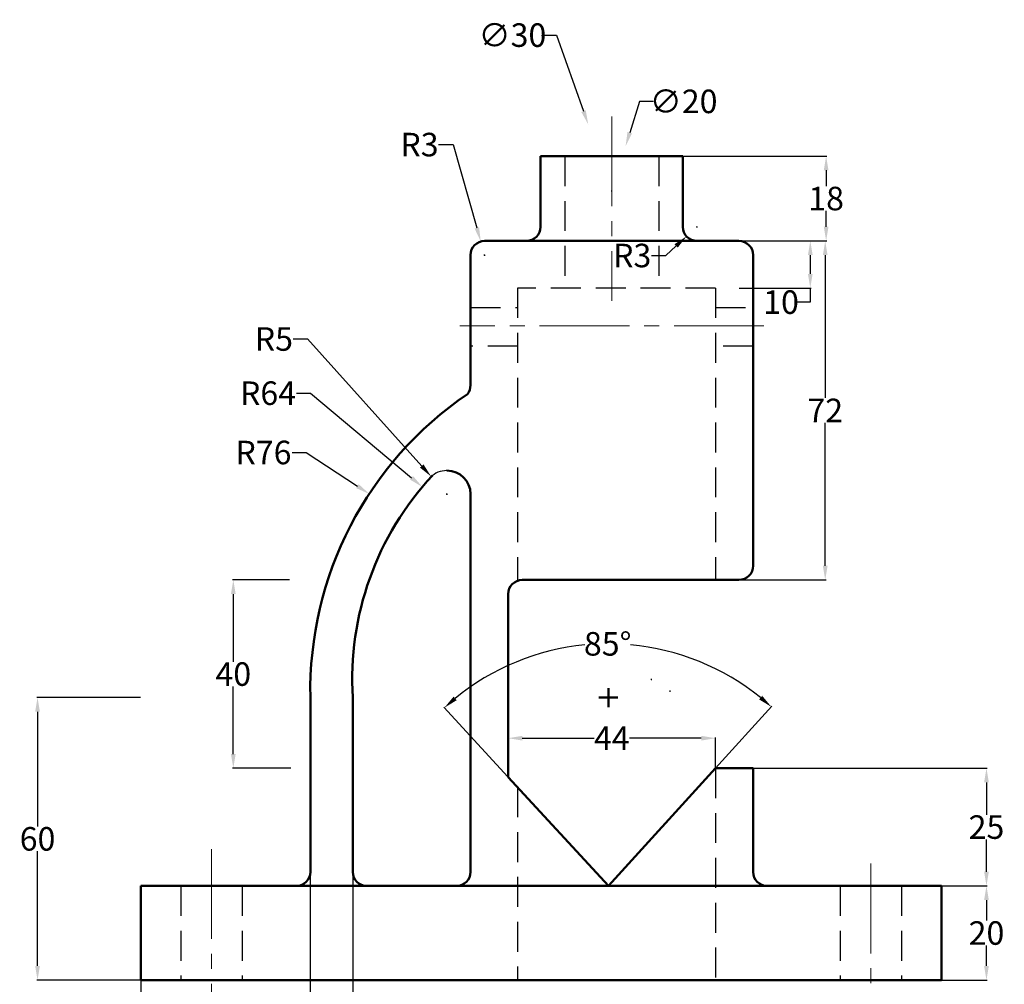
# Model space of a CAD drawing. Units: metres. Extents: x -2793 to -2360, y -31 to 491.
# Tile 2 of 4: x -2786 to -2577, y 144 to 349. Entities that reach past the tile are written whole.
import ezdxf

# ---------------------------------------------------------------- set-up
doc = ezdxf.new("R2010")
doc.units = ezdxf.units.M
doc.linetypes.add('CENTER2', pattern=[28.575, 19.05, -3.175, 3.175, -3.175])
doc.linetypes.add('DASHED2', pattern=[9.525, 6.35, -3.175])
for name, color, linetype, lineweight in [('M-CNTR', 9, 'CENTER2', 18), ('M-DIMS', 2, 'Continuous', 25), ('M-HIDN', 9, 'DASHED2', 25), ('M-OUTL', 7, 'Continuous', 50)]:
    doc.layers.add(name, color=color, linetype=linetype, lineweight=lineweight)
doc.styles.get("Standard").update_dxf_attribs({"font": 'arial.ttf'})
doc.dimstyles.get("Standard").update_dxf_attribs({"dimtxt": 5, "dimasz": 3, "dimexe": 0.18, "dimexo": 0.0625, "dimgap": 0.09, "dimtad": 0, "dimtih": 1, "dimtoh": 1, "dimdec": 0, "dimzin": 0, "dimdsep": 46, "dimtxsty": 'Standard', "dimcen": 0.09, "dimclrd": 254, "dimclre": 254, "dimadec": 0, "dimazin": 0, "dimtfac": 1, "dimtdec": 0, "dimtofl": 0, "dimtmove": 0, "dimatfit": 3, "dimfxl": 1, "dimtolj": 1, "dimtzin": 0, "dimarcsym": 0})

# ---------------------------------------------------------------- blocks, each defined once
blk = doc.blocks.new('*D15')
at = {"layer": 'Defpoints', "color": 0, "transparency": 16777216}
for p in [(-2648.17, 215.08), (-2681.87, 188.31), (-2637.87, 190.18), (-2660.6, 165.18), (-2660.6, 165.18)]:
    blk.add_point(p, dxfattribs=at)
at = {"layer": 'M-DIMS', "color": 0, "lineweight": -2, "transparency": 16777216}
for p, q in [((-2681.91, 188.36), (-2695.53, 203.17)), ((-2637.83, 190.22), (-2625.88, 203.36))]:
    blk.add_line(p, q, dxfattribs=at)
for start, end in [(95.5587, 129.2471), (51.0616, 84.7514)]:
    blk.add_arc((-2660.6, 165.18), 51.43, start, end, dxfattribs=at)
at = {"layer": 'M-DIMS', "color": 0, "transparency": 16777216}
for points in [[(-2692.81, 204.62), (-2693.47, 205.38), (-2695.4, 203.04)], [(-2627.95, 205.56), (-2628.6, 204.8), (-2626, 203.22)]]:
    blk.add_solid(points, dxfattribs=at)
at = {"layer": 'M-DIMS', "color": 0, "transparency": 16777216, "insert": (-2660.74, 216.6), "char_height": 5, "attachment_point": 5}
blk.add_mtext('\\A1;{\\fTimes New Roman|b0|i0|c0|p18;85°}', dxfattribs=at)
blk = doc.blocks.new('*D16')
at = {"layer": 'Defpoints', "color": 0, "transparency": 16777216}
for p in [(-2781.78, 205.18), (-2759.87, 205.18), (-2759.87, 145.18)]:
    blk.add_point(p, dxfattribs=at)
at = {"layer": 'M-DIMS', "color": 0, "lineweight": -2, "transparency": 16777216}
for p, q in [((-2759.93, 205.18), (-2781.96, 205.18)), ((-2781.78, 202.18), (-2781.78, 177.81)), ((-2781.78, 148.18), (-2781.78, 172.54)), ((-2759.93, 145.18), (-2781.96, 145.18))]:
    blk.add_line(p, q, dxfattribs=at)
at = {"layer": 'M-DIMS', "color": 0, "transparency": 16777216}
for points in [[(-2782.28, 202.18), (-2781.28, 202.18), (-2781.78, 205.18)], [(-2782.28, 148.18), (-2781.28, 148.18), (-2781.78, 145.18)]]:
    blk.add_solid(points, dxfattribs=at)
at = {"layer": 'M-DIMS', "color": 0, "transparency": 16777216, "insert": (-2781.78, 175.18), "char_height": 5, "attachment_point": 5}
blk.add_mtext('\\A1;{\\fTimes New Roman|b0|i0|c0|p18;60}', dxfattribs=at)
blk = doc.blocks.new('*D17')
at = {"layer": 'Defpoints', "color": 0, "transparency": 16777216}
for p in [(-2656.94, 322.3), (-2662.8, 303.26)]:
    blk.add_point(p, dxfattribs=at)
at = {"layer": 'M-DIMS', "color": 0, "lineweight": -2, "transparency": 16777216}
for p, q in [((-2654.01, 331.82), (-2656.06, 325.17)), ((-2651.01, 331.82), (-2654.01, 331.82)), ((-2659.96, 312.78), (-2659.78, 312.78)), ((-2659.87, 312.69), (-2659.87, 312.87))]:
    blk.add_line(p, q, dxfattribs=at)
at = {"layer": 'M-DIMS', "color": 0, "transparency": 16777216}
blk.add_solid([(-2656.54, 325.32), (-2655.58, 325.02), (-2656.94, 322.3)], dxfattribs=at)
at = {"layer": 'M-DIMS', "color": 0, "transparency": 16777216, "insert": (-2644.63, 331.82), "char_height": 5, "attachment_point": 5}
blk.add_mtext('\\A1;∅20', dxfattribs=at)
blk = doc.blocks.new('*D18')
at = {"layer": 'Defpoints', "color": 0, "transparency": 16777216}
for p in [(-2664.87, 326.92), (-2654.87, 298.64)]:
    blk.add_point(p, dxfattribs=at)
at = {"layer": 'M-DIMS', "color": 0, "lineweight": -2, "transparency": 16777216}
for p, q in [((-2674.78, 345.89), (-2671.58, 345.89)), ((-2671.58, 345.89), (-2665.87, 329.75)), ((-2659.96, 312.78), (-2659.78, 312.78)), ((-2659.87, 312.69), (-2659.87, 312.87))]:
    blk.add_line(p, q, dxfattribs=at)
at = {"layer": 'M-DIMS', "color": 0, "transparency": 16777216}
blk.add_solid([(-2665.4, 329.91), (-2666.34, 329.58), (-2664.87, 326.92)], dxfattribs=at)
at = {"layer": 'M-DIMS', "color": 0, "transparency": 16777216, "insert": (-2680.97, 345.89), "char_height": 5, "attachment_point": 5}
blk.add_mtext('\\A1;{\\fTimes New Roman|b0|i0|c0|p18;∅30}', dxfattribs=at)
blk = doc.blocks.new('*D19')
at = {"layer": 'Defpoints', "color": 0, "transparency": 16777216}
for p in [(-2687.69, 302.06), (-2686.87, 299.18)]:
    blk.add_point(p, dxfattribs=at)
at = {"layer": 'M-DIMS', "color": 0, "lineweight": -2, "transparency": 16777216}
for p, q in [((-2696.67, 322.64), (-2693.57, 322.64)), ((-2693.57, 322.64), (-2688.52, 304.94)), ((-2686.96, 299.18), (-2686.78, 299.18)), ((-2686.87, 299.09), (-2686.87, 299.27))]:
    blk.add_line(p, q, dxfattribs=at)
at = {"layer": 'M-DIMS', "color": 0, "transparency": 16777216}
blk.add_solid([(-2688.04, 305.08), (-2689, 304.81), (-2687.69, 302.06)], dxfattribs=at)
at = {"layer": 'M-DIMS', "color": 0, "transparency": 16777216, "insert": (-2700.7, 322.64), "char_height": 5, "attachment_point": 5}
blk.add_mtext('\\A1;{\\fTimes New Roman|b0|i0|c0|p18;R3}', dxfattribs=at)
blk = doc.blocks.new('*D20')
at = {"layer": 'Defpoints', "color": 0, "transparency": 16777216}
for p in [(-2698.21, 252.13), (-2694.87, 248.41)]:
    blk.add_point(p, dxfattribs=at)
at = {"layer": 'M-DIMS', "color": 0, "lineweight": -2, "transparency": 16777216}
for p, q in [((-2727.52, 281.35), (-2724.47, 281.35)), ((-2724.47, 281.35), (-2700.21, 254.36)), ((-2694.96, 248.41), (-2694.78, 248.41)), ((-2694.87, 248.32), (-2694.87, 248.5))]:
    blk.add_line(p, q, dxfattribs=at)
blk.add_arc((-2694.87, 248.41), 5, 90.7162, 134.0032, dxfattribs=at)
at = {"layer": 'M-DIMS', "color": 0, "transparency": 16777216}
blk.add_solid([(-2699.84, 254.7), (-2700.59, 254.03), (-2698.21, 252.13)], dxfattribs=at)
at = {"layer": 'M-DIMS', "color": 0, "transparency": 16777216, "insert": (-2731.61, 281.35), "char_height": 5, "attachment_point": 5}
blk.add_mtext('\\A1;{\\fTimes New Roman|b0|i0|c0|p18;R5}', dxfattribs=at)
blk = doc.blocks.new('*D21')
at = {"layer": 'Defpoints', "color": 0, "transparency": 16777216}
for p in [(-2711.37, 248.45), (-2647.51, 206.57)]:
    blk.add_point(p, dxfattribs=at)
at = {"layer": 'M-DIMS', "color": 0, "lineweight": -2, "transparency": 16777216}
for p, q in [((-2727.76, 257.24), (-2724.76, 257.24)), ((-2724.76, 257.24), (-2713.88, 250.1)), ((-2647.6, 206.57), (-2647.42, 206.57)), ((-2647.51, 206.48), (-2647.51, 206.66))]:
    blk.add_line(p, q, dxfattribs=at)
at = {"layer": 'M-DIMS', "color": 0, "transparency": 16777216}
blk.add_solid([(-2713.6, 250.52), (-2714.15, 249.68), (-2711.37, 248.45)], dxfattribs=at)
at = {"layer": 'M-DIMS', "color": 0, "transparency": 16777216, "insert": (-2733.82, 257.24), "char_height": 5, "attachment_point": 5}
blk.add_mtext('\\A1;R76', dxfattribs=at)
blk = doc.blocks.new('*D22')
at = {"layer": 'Defpoints', "color": 0, "transparency": 16777216}
for p in [(-2700.09, 249.93), (-2651.44, 209.05)]:
    blk.add_point(p, dxfattribs=at)
at = {"layer": 'M-DIMS', "color": 0, "lineweight": -2, "transparency": 16777216}
for p, q in [((-2726.8, 269.84), (-2723.8, 269.84)), ((-2723.8, 269.84), (-2702.39, 251.86)), ((-2651.53, 209.05), (-2651.35, 209.05)), ((-2651.44, 208.96), (-2651.44, 209.14))]:
    blk.add_line(p, q, dxfattribs=at)
at = {"layer": 'M-DIMS', "color": 0, "transparency": 16777216}
blk.add_solid([(-2702.07, 252.24), (-2702.71, 251.48), (-2700.09, 249.93)], dxfattribs=at)
at = {"layer": 'M-DIMS', "color": 0, "transparency": 16777216, "insert": (-2732.85, 269.84), "char_height": 5, "attachment_point": 5}
blk.add_mtext('\\A1;R64', dxfattribs=at)
blk = doc.blocks.new('*D23')
at = {"layer": 'Defpoints', "color": 0, "transparency": 16777216}
for p in [(-2728.24, 230.18), (-2740.22, 190.18), (-2727.94, 190.18)]:
    blk.add_point(p, dxfattribs=at)
at = {"layer": 'M-DIMS', "color": 0, "lineweight": -2, "transparency": 16777216}
for p, q in [((-2728.3, 230.18), (-2740.4, 230.18)), ((-2740.22, 227.18), (-2740.22, 212.81)), ((-2740.22, 193.18), (-2740.22, 207.54)), ((-2728, 190.18), (-2740.4, 190.18))]:
    blk.add_line(p, q, dxfattribs=at)
at = {"layer": 'M-DIMS', "color": 0, "transparency": 16777216}
for points in [[(-2740.72, 227.18), (-2739.72, 227.18), (-2740.22, 230.18)], [(-2740.72, 193.18), (-2739.72, 193.18), (-2740.22, 190.18)]]:
    blk.add_solid(points, dxfattribs=at)
at = {"layer": 'M-DIMS', "color": 0, "transparency": 16777216, "insert": (-2740.22, 210.18), "char_height": 5, "attachment_point": 5}
blk.add_mtext('\\A1;{\\fTimes New Roman|b0|i0|c0|p18;40}', dxfattribs=at)
blk = doc.blocks.new('*D24')
at = {"layer": 'Defpoints', "color": 0, "transparency": 16777216}
for p in [(-2681.87, 196.56), (-2681.87, 188.31), (-2637.87, 190.18)]:
    blk.add_point(p, dxfattribs=at)
at = {"layer": 'M-DIMS', "color": 0, "lineweight": -2, "transparency": 16777216}
for p, q in [((-2681.87, 188.37), (-2681.87, 196.74)), ((-2678.87, 196.56), (-2663.63, 196.56)), ((-2640.87, 196.56), (-2656.11, 196.56)), ((-2637.87, 190.24), (-2637.87, 196.74))]:
    blk.add_line(p, q, dxfattribs=at)
at = {"layer": 'M-DIMS', "color": 0, "transparency": 16777216}
for points in [[(-2678.87, 197.06), (-2678.87, 196.06), (-2681.87, 196.56)], [(-2640.87, 197.06), (-2640.87, 196.06), (-2637.87, 196.56)]]:
    blk.add_solid(points, dxfattribs=at)
at = {"layer": 'M-DIMS', "color": 0, "transparency": 16777216, "insert": (-2659.87, 196.56), "char_height": 5, "attachment_point": 5}
blk.add_mtext('\\A1;44', dxfattribs=at)
blk = doc.blocks.new('*D25')
at = {"layer": 'Defpoints', "color": 0, "transparency": 16777216}
for p in [(-2589.87, 165.18), (-2589.87, 145.18), (-2580.33, 145.18)]:
    blk.add_point(p, dxfattribs=at)
at = {"layer": 'M-DIMS', "color": 0, "lineweight": -2, "transparency": 16777216}
for p, q in [((-2589.81, 165.18), (-2580.15, 165.18)), ((-2580.33, 162.18), (-2580.33, 157.81)), ((-2580.33, 148.18), (-2580.33, 152.54)), ((-2589.81, 145.18), (-2580.15, 145.18))]:
    blk.add_line(p, q, dxfattribs=at)
at = {"layer": 'M-DIMS', "color": 0, "transparency": 16777216}
for points in [[(-2580.83, 162.18), (-2579.83, 162.18), (-2580.33, 165.18)], [(-2580.83, 148.18), (-2579.83, 148.18), (-2580.33, 145.18)]]:
    blk.add_solid(points, dxfattribs=at)
at = {"layer": 'M-DIMS', "color": 0, "transparency": 16777216, "insert": (-2580.33, 155.18), "char_height": 5, "attachment_point": 5}
blk.add_mtext('\\A1;{\\fTimes New Roman|b0|i0|c0|p18;20}', dxfattribs=at)
blk = doc.blocks.new('*D26')
at = {"layer": 'Defpoints', "color": 0, "transparency": 16777216}
for p in [(-2629.87, 190.18), (-2629.87, 165.18), (-2580.33, 165.18)]:
    blk.add_point(p, dxfattribs=at)
at = {"layer": 'M-DIMS', "color": 0, "lineweight": -2, "transparency": 16777216}
for p, q in [((-2629.81, 190.18), (-2580.15, 190.18)), ((-2580.33, 187.18), (-2580.33, 180.31)), ((-2580.33, 168.18), (-2580.33, 175.04)), ((-2629.81, 165.18), (-2580.15, 165.18))]:
    blk.add_line(p, q, dxfattribs=at)
at = {"layer": 'M-DIMS', "color": 0, "transparency": 16777216}
for points in [[(-2580.83, 187.18), (-2579.83, 187.18), (-2580.33, 190.18)], [(-2580.83, 168.18), (-2579.83, 168.18), (-2580.33, 165.18)]]:
    blk.add_solid(points, dxfattribs=at)
at = {"layer": 'M-DIMS', "color": 0, "transparency": 16777216, "insert": (-2580.33, 177.68), "char_height": 5, "attachment_point": 5}
blk.add_mtext('\\A1;{\\fTimes New Roman|b0|i0|c0|p18;25}', dxfattribs=at)
blk = doc.blocks.new('*D27')
at = {"layer": 'Defpoints', "color": 0, "transparency": 16777216}
for p in [(-2632.87, 302.18), (-2632.87, 292.18), (-2617.73, 292.18)]:
    blk.add_point(p, dxfattribs=at)
at = {"layer": 'M-DIMS', "color": 0, "lineweight": -2, "transparency": 16777216}
for p, q in [((-2632.81, 302.18), (-2617.55, 302.18)), ((-2617.73, 299.18), (-2617.73, 295.18)), ((-2632.81, 292.18), (-2617.55, 292.18)), ((-2617.73, 292.18), (-2617.73, 289.18)), ((-2617.73, 289.18), (-2620.73, 289.18))]:
    blk.add_line(p, q, dxfattribs=at)
at = {"layer": 'M-DIMS', "color": 0, "transparency": 16777216}
for points in [[(-2618.23, 299.18), (-2617.23, 299.18), (-2617.73, 302.18)], [(-2618.23, 295.18), (-2617.23, 295.18), (-2617.73, 292.18)]]:
    blk.add_solid(points, dxfattribs=at)
at = {"layer": 'M-DIMS', "color": 0, "transparency": 16777216, "insert": (-2623.94, 289.18), "char_height": 5, "attachment_point": 5}
blk.add_mtext('\\A1;{\\fTimes New Roman|b0|i0|c0|p18;10}', dxfattribs=at)
blk = doc.blocks.new('*D28')
at = {"layer": 'Defpoints', "color": 0, "transparency": 16777216}
for p in [(-2644.8, 320.18), (-2644.8, 302.18), (-2614.37, 302.18)]:
    blk.add_point(p, dxfattribs=at)
at = {"layer": 'M-DIMS', "color": 0, "lineweight": -2, "transparency": 16777216}
for p, q in [((-2644.74, 320.18), (-2614.19, 320.18)), ((-2614.37, 317.18), (-2614.37, 313.81)), ((-2614.37, 305.18), (-2614.37, 308.54)), ((-2644.74, 302.18), (-2614.19, 302.18))]:
    blk.add_line(p, q, dxfattribs=at)
at = {"layer": 'M-DIMS', "color": 0, "transparency": 16777216}
for points in [[(-2614.87, 317.18), (-2613.87, 317.18), (-2614.37, 320.18)], [(-2614.87, 305.18), (-2613.87, 305.18), (-2614.37, 302.18)]]:
    blk.add_solid(points, dxfattribs=at)
at = {"layer": 'M-DIMS', "color": 0, "transparency": 16777216, "insert": (-2614.37, 311.18), "char_height": 5, "attachment_point": 5}
blk.add_mtext('\\A1;{\\fTimes New Roman|b0|i0|c0|p18;18}', dxfattribs=at)
blk = doc.blocks.new('*D29')
at = {"layer": 'Defpoints', "color": 0, "transparency": 16777216}
for p in [(-2632.87, 302.18), (-2632.87, 230.18), (-2614.56, 230.18)]:
    blk.add_point(p, dxfattribs=at)
at = {"layer": 'M-DIMS', "color": 0, "lineweight": -2, "transparency": 16777216}
for p, q in [((-2632.81, 302.18), (-2614.38, 302.18)), ((-2614.56, 299.18), (-2614.56, 268.82)), ((-2614.56, 233.18), (-2614.56, 263.53)), ((-2632.81, 230.18), (-2614.38, 230.18))]:
    blk.add_line(p, q, dxfattribs=at)
at = {"layer": 'M-DIMS', "color": 0, "transparency": 16777216}
for points in [[(-2615.06, 299.18), (-2614.06, 299.18), (-2614.56, 302.18)], [(-2615.06, 233.18), (-2614.06, 233.18), (-2614.56, 230.18)]]:
    blk.add_solid(points, dxfattribs=at)
at = {"layer": 'M-DIMS', "color": 0, "transparency": 16777216, "insert": (-2614.56, 266.18), "char_height": 5, "attachment_point": 5}
blk.add_mtext('\\A1;{\\fTimes New Roman|b0|i0|c0|p18;72}', dxfattribs=at)
blk = doc.blocks.new('*D56')
at = {"layer": 'Defpoints', "color": 0, "transparency": 16777216}
for p in [(-2723.87, 168.18), (-2759.87, 145.18), (-2723.87, 121.23)]:
    blk.add_point(p, dxfattribs=at)
at = {"layer": 'M-DIMS', "color": 254, "lineweight": -2, "transparency": 16777216}
for p, q in [((-2723.87, 168.11), (-2723.87, 121.05)), ((-2759.87, 145.11), (-2759.87, 121.05)), ((-2756.87, 121.23), (-2745.54, 121.23)), ((-2726.87, 121.23), (-2738.2, 121.23))]:
    blk.add_line(p, q, dxfattribs=at)
at = {"layer": 'M-DIMS', "color": 254, "transparency": 16777216}
for points in [[(-2756.87, 121.73), (-2756.87, 120.73), (-2759.87, 121.23)], [(-2726.87, 121.73), (-2726.87, 120.73), (-2723.87, 121.23)]]:
    blk.add_solid(points, dxfattribs=at)
at = {"layer": 'M-DIMS', "color": 0, "transparency": 16777216, "insert": (-2741.87, 121.23), "char_height": 5, "attachment_point": 5}
blk.add_mtext('\\A1;36', dxfattribs=at)
blk = doc.blocks.new('*D57')
at = {"layer": 'Defpoints', "color": 0, "transparency": 16777216}
for p in [(-2723.87, 168.18), (-2714.87, 168.18), (-2714.87, 121.23)]:
    blk.add_point(p, dxfattribs=at)
at = {"layer": 'M-DIMS', "color": 254, "lineweight": -2, "transparency": 16777216}
for p, q in [((-2723.87, 168.11), (-2723.87, 121.05)), ((-2714.87, 168.11), (-2714.87, 121.05)), ((-2720.87, 121.23), (-2717.87, 121.23)), ((-2714.87, 121.23), (-2711.87, 121.23))]:
    blk.add_line(p, q, dxfattribs=at)
at = {"layer": 'M-DIMS', "color": 254, "transparency": 16777216}
for points in [[(-2720.87, 121.73), (-2720.87, 120.73), (-2723.87, 121.23)], [(-2717.87, 121.73), (-2717.87, 120.73), (-2714.87, 121.23)]]:
    blk.add_solid(points, dxfattribs=at)
at = {"layer": 'M-DIMS', "color": 0, "transparency": 16777216, "insert": (-2710.13, 121.23), "char_height": 5, "attachment_point": 5}
blk.add_mtext('\\A1;9', dxfattribs=at)
blk = doc.blocks.new('*D68')
at = {"layer": 'Defpoints', "color": 0, "transparency": 16777216}
for p in [(-2641.8, 305.18), (-2644.01, 303.15)]:
    blk.add_point(p, dxfattribs=at)
at = {"layer": 'M-DIMS', "color": 254, "lineweight": -2, "transparency": 16777216}
for p, q in [((-2641.89, 305.18), (-2641.71, 305.18)), ((-2641.8, 305.09), (-2641.8, 305.27)), ((-2648.42, 299.08), (-2646.21, 301.11)), ((-2651.42, 299.08), (-2648.42, 299.08))]:
    blk.add_line(p, q, dxfattribs=at)
at = {"layer": 'M-DIMS', "color": 254, "transparency": 16777216}
blk.add_solid([(-2646.55, 301.48), (-2645.88, 300.75), (-2644.01, 303.15)], dxfattribs=at)
at = {"layer": 'M-DIMS', "color": 0, "transparency": 16777216, "insert": (-2655.54, 299.08), "char_height": 5, "attachment_point": 5}
blk.add_mtext('\\A1;R3', dxfattribs=at)

msp = doc.modelspace()

# ---------------------------------------------------------------- linework, layer by layer
at = {"layer": 'M-CNTR'}
for p, q in [((-2659.868, 328.595), (-2659.868, 289.42)), ((-2627.566, 284.142), (-2692.115, 284.142)), ((-2744.868, 172.975), (-2744.868, 136.879)), ((-2604.868, 169.913), (-2604.868, 140.718))]:
    msp.add_line(p, q, dxfattribs=at)
at = {"layer": 'M-HIDN'}
for p, q in [((-2669.868, 320.175), (-2669.868, 292.175)), ((-2649.868, 320.175), (-2649.868, 292.175)), ((-2637.868, 292.175), (-2679.868, 292.175)), ((-2679.868, 292.175), (-2679.868, 230.004)), ((-2637.868, 292.175), (-2637.868, 230.175)), ((-2689.868, 288.016), (-2679.868, 288.016)), ((-2637.868, 288.016), (-2629.868, 288.016)), ((-2679.868, 279.796), (-2689.868, 279.796)), ((-2629.868, 279.796), (-2637.868, 279.796)), ((-2637.868, 190.175), (-2637.868, 145.175)), ((-2679.868, 186.135), (-2679.868, 145.175)), ((-2751.368, 165.175), (-2751.368, 145.175)), ((-2738.368, 165.175), (-2738.368, 145.175)), ((-2611.368, 165.175), (-2611.368, 145.175)), ((-2598.368, 165.175), (-2598.368, 145.175))]:
    msp.add_line(p, q, dxfattribs=at)
at = {"layer": 'M-OUTL'}
for p, q in [((-2644.798, 320.175), (-2674.999, 320.175)), ((-2674.999, 320.175), (-2674.999, 305.175)), ((-2644.798, 320.175), (-2644.798, 305.175)), ((-2677.999, 302.175), (-2686.868, 302.175)), ((-2677.999, 302.175), (-2641.798, 302.175)), ((-2632.868, 302.175), (-2641.798, 302.175)), ((-2689.868, 299.175), (-2689.868, 271.546)), ((-2629.868, 299.175), (-2629.868, 233.175)), ((-2689.868, 248.411), (-2689.868, 168.175)), ((-2632.868, 230.175), (-2678.868, 230.175)), ((-2681.868, 227.175), (-2681.868, 188.311)), ((-2660.601, 205.175), (-2660.601, 207.175)), ((-2660.601, 207.175), (-2660.601, 203.175)), ((-2723.868, 205.175), (-2723.868, 168.175)), ((-2714.868, 205.175), (-2714.868, 168.175)), ((-2658.601, 205.175), (-2662.601, 205.175)), ((-2660.601, 205.175), (-2658.601, 205.175)), ((-2681.868, 188.311), (-2660.601, 165.175)), ((-2660.601, 165.175), (-2637.868, 190.175)), ((-2629.868, 190.175), (-2637.868, 190.175)), ((-2629.868, 190.175), (-2629.868, 168.175)), ((-2759.868, 165.175), (-2759.868, 145.175)), ((-2726.868, 165.175), (-2759.868, 165.175)), ((-2726.868, 165.175), (-2711.868, 165.175)), ((-2692.868, 165.175), (-2711.868, 165.175)), ((-2626.868, 165.175), (-2692.868, 165.175)), ((-2589.868, 165.175), (-2626.868, 165.175)), ((-2589.868, 145.175), (-2589.868, 165.175)), ((-2759.868, 145.175), (-2589.868, 145.175))]:
    msp.add_line(p, q, dxfattribs=at)
for centre, radius, start, end in [((-2677.999, 305.175), 3, 270, 0), ((-2641.798, 305.175), 3, 180, 270), ((-2686.868, 299.175), 3, 90, 180), ((-2632.868, 299.175), 3, 360, 90), ((-2647.512, 206.565), 76.368, 124.2849, 181.04273), ((-2692.868, 271.546), 3, 321.16359, 0), ((-2694.868, 248.411), 5, 0, 90), ((-2651.44, 209.05), 63.546, 137.06049, 183.4962), ((-2632.868, 233.175), 3, 270, 360), ((-2678.868, 227.175), 3, 90, 180), ((-2726.868, 168.175), 3, 270, 0), ((-2711.868, 168.175), 3, 180, 270), ((-2692.868, 168.175), 3, 270, 0), ((-2626.868, 168.175), 3, 180, 270)]:
    msp.add_arc(centre, radius, start, end, dxfattribs=at)

# ---------------------------------------------------------------- dimensions: what is measured, and where the dimension line sits
at = {"layer": 'M-DIMS'}
dim = msp.add_diameter_dim_2p(p1=(-2654.866, 298.643), p2=(-2664.87, 326.918), text='{\\fTimes New Roman|b0|i0|c0|p18;<>}', dimstyle='Standard', override={"dimclrd": 0, "dimclre": 0, "dimclrt": 0}, dxfattribs=at)
dim.commit()
dim.dimension.update_dxf_attribs({"geometry": '*D18', "text_midpoint": (-2680.965, 345.89), "dimtype": 163})
dim = msp.add_diameter_dim_2p(p1=(-2662.796, 303.26), p2=(-2656.94, 322.302), dimstyle='Standard', override={"dimclrd": 0, "dimclre": 0, "dimclrt": 0}, dxfattribs=at)
dim.commit()
dim.dimension.update_dxf_attribs({"geometry": '*D17', "text_midpoint": (-2644.631, 331.817), "dimtype": 163})
for center, mpoint, picture, middle in [((-2686.868, 299.175), (-2687.692, 302.06), '*D19', (-2700.696, 322.642)), ((-2694.868, 248.411), (-2698.209, 252.13), '*D20', (-2731.606, 281.352))]:
    dim = msp.add_radius_dim(center=center, mpoint=mpoint, text='{\\fTimes New Roman|b0|i0|c0|p18;<>}', dimstyle='Standard', override={"dimclrd": 0, "dimclre": 0, "dimclrt": 0}, dxfattribs=at)
    dim.commit()
    dim.dimension.update_dxf_attribs({"geometry": picture, "text_midpoint": middle, "dimtype": 164})
for base, p1, p2, picture, middle in [((-2614.366, 302.175), (-2644.798, 320.175), (-2644.798, 302.175), '*D28', (-2614.366, 311.175)), ((-2617.726, 292.175), (-2632.868, 302.175), (-2632.868, 292.175), '*D27', (-2623.944, 289.175)), ((-2614.559, 230.175), (-2632.868, 302.175), (-2632.868, 230.175), '*D29', (-2614.559, 266.175)), ((-2740.216, 190.175), (-2728.24, 230.175), (-2727.941, 190.175), '*D23', (-2740.216, 210.175)), ((-2781.782, 205.175), (-2759.868, 145.175), (-2759.868, 205.175), '*D16', (-2781.782, 175.175)), ((-2580.331, 165.175), (-2629.868, 190.175), (-2629.868, 165.175), '*D26', (-2580.331, 177.675)), ((-2580.331, 145.175), (-2589.868, 165.175), (-2589.868, 145.175), '*D25', (-2580.331, 155.175))]:
    dim = msp.add_linear_dim(base=base, p1=p1, p2=p2, angle=90, text='{\\fTimes New Roman|b0|i0|c0|p18;<>}', dimstyle='Standard', override={"dimclrd": 0, "dimclre": 0, "dimclrt": 0}, dxfattribs=at)
    dim.commit()
    dim.dimension.update_dxf_attribs({"geometry": picture, "text_midpoint": middle})
dim = msp.add_radius_dim(center=(-2641.798, 305.175), mpoint=(-2644.006, 303.145), dimstyle='Standard', override={"dimdec": 0, "dimlfac": 1, "dimrnd": 0, "dimzin": 0, "dimdsep": 46, "dimlunit": 2}, dxfattribs=at)
dim.commit()
dim.dimension.update_dxf_attribs({"geometry": '*D68', "text_midpoint": (-2655.545, 299.084)})
for center, mpoint, picture, middle in [((-2651.44, 209.05), (-2700.093, 249.928), '*D22', (-2732.849, 269.844)), ((-2647.512, 206.565), (-2711.368, 248.452), '*D21', (-2733.82, 257.235))]:
    dim = msp.add_radius_dim(center=center, mpoint=mpoint, dimstyle='Standard', override={"dimclrd": 0, "dimclre": 0, "dimclrt": 0}, dxfattribs=at)
    dim.commit()
    dim.dimension.update_dxf_attribs({"geometry": picture, "text_midpoint": middle, "dimtype": 164})
dim = msp.add_angular_dim_2l(base=(-2648.167, 215.078), line1=((-2681.868, 188.311), (-2660.601, 165.175)), line2=((-2660.601, 165.175), (-2637.868, 190.175)), text='{\\fTimes New Roman|b0|i0|c0|p18;<>}', dimstyle='Standard', override={"dimclrd": 0, "dimclre": 0, "dimclrt": 0}, dxfattribs=at)
dim.commit()
dim.dimension.update_dxf_attribs({"geometry": '*D15', "text_midpoint": (-2660.739, 216.603)})
for base, p1, p2, override, picture, middle in [((-2681.868, 196.558), (-2637.868, 190.175), (-2681.868, 188.311), {"dimclrd": 0, "dimclre": 0, "dimclrt": 0}, '*D24', (-2659.868, 196.558)), ((-2723.868, 121.229), (-2759.868, 145.175), (-2723.868, 168.175), {"dimdec": 0, "dimlfac": 1, "dimrnd": 0, "dimzin": 0, "dimdsep": 46, "dimlunit": 2}, '*D56', (-2741.868, 121.229)), ((-2714.868, 121.229), (-2723.868, 168.175), (-2714.868, 168.175), {"dimdec": 0, "dimlfac": 1, "dimrnd": 0, "dimzin": 0, "dimdsep": 46, "dimlunit": 2}, '*D57', (-2710.134, 121.229))]:
    dim = msp.add_linear_dim(base=base, p1=p1, p2=p2, dimstyle='Standard', override=override, dxfattribs=at)
    dim.commit()
    dim.dimension.update_dxf_attribs({"geometry": picture, "text_midpoint": middle})

doc.saveas('drawing.dxf')
